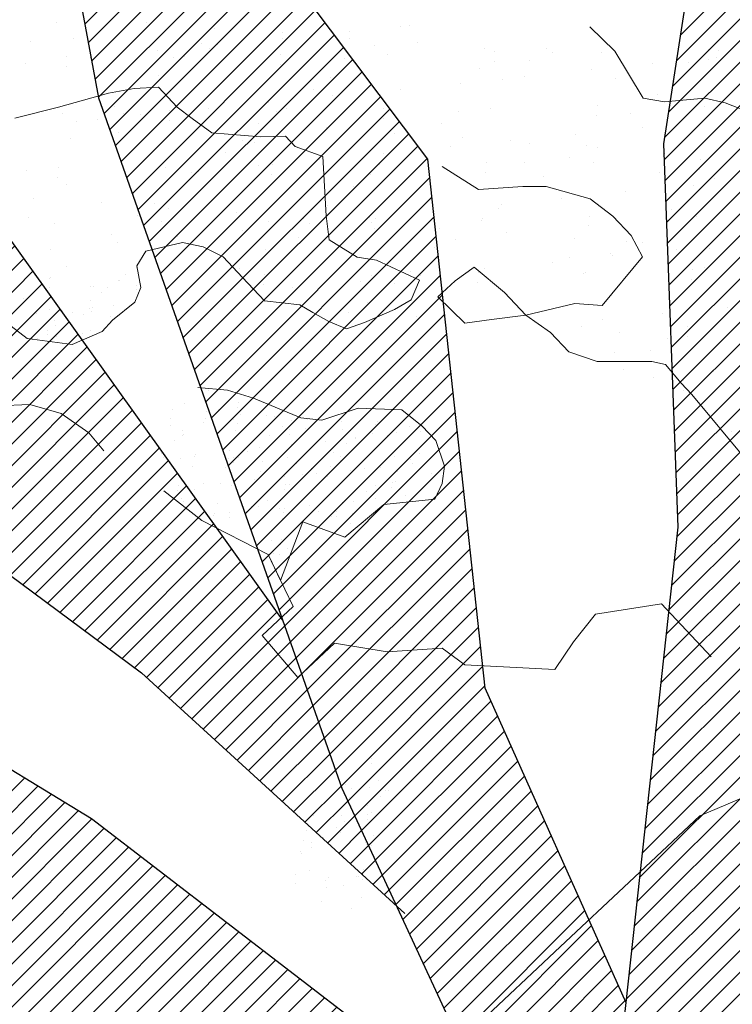
# Model space of a CAD drawing. Units: inches. Extents: x 1986 to 21484, y -1816 to 2016.
# Tile 72 of 85: x 3662.33 to 3669.485, y 1888.787 to 1898.672. Entities that reach past the tile are written whole.
import ezdxf

# ---------------------------------------------------------------- set-up
doc = ezdxf.new("R2010")
doc.units = ezdxf.units.IN
doc.layers.add('L-PLNT', color=84, linetype='Continuous', lineweight=13)
doc.layers.add('vfolhas', color=114, linetype='Continuous', lineweight=5)
doc.layers.add('vfolha2', color=110, linetype='Continuous')
doc.layers.add('vfolhas2', color=102, linetype='Continuous')
pattern_1 = [(45, (-2446.5133113, 50.986076), (-0.004419417382, 0.004419417382), [])]

# ---------------------------------------------------------------- blocks, each defined once
blk = doc.blocks.new('arbusto_PB_verde_grande')
at = {"layer": 'vfolha2'}
h = blk.add_hatch(dxfattribs=at)
h.set_pattern_fill('ANSI31', color=256, scale=0.05, style=0)
h.set_pattern_definition(pattern_1)
h.paths.add_polyline_path([(0.02944, 0.35651), (0.00028, 0.09048), (0.02625, -0.03934), (0.047, 0.06233), (0.06189, 0.09731), (0.09372, 0.26573), (0.09955, 0.43473), (0.08789, 0.61313), (0.0645, 0.72266), (0.04988, 0.6851), (0.0236, 0.51294)])
h.paths.add_polyline_path([(0.30106, 0.43789), (0.14225, 0.24871), (0.26685, 0.30022)])
h.paths.add_polyline_path([(0.37995, 0.22817), (0.23697, 0.15193), (0.18428, 0.09364), (0.11122, 0.04358), (0.02625, -0.03934), (0.28061, 0.04667), (0.36829, 0.07798), (0.46756, 0.11239), (0.61068, 0.19376), (0.71585, 0.27823), (0.55813, 0.25948)])
h.paths.add_polyline_path([(0.56101, -0.29441), (0.72752, -0.32573), (0.59024, -0.2412), (0.42962, -0.15982), (0.02625, -0.03934), (0.14922, -0.14107), (0.18838, -0.16604), (0.41501, -0.24435)])
h.paths.add_polyline_path([(-0.27429, -0.44776), (-0.30352, -0.72628), (-0.23923, -0.64175), (-0.15457, -0.45716), (0.02625, -0.03934), (-0.16328, -0.25376)])
h.paths.add_polyline_path([(-0.51963, -0.24744), (-0.67736, -0.32573), (-0.59558, -0.35072), (-0.40574, -0.32882), (-0.21007, -0.20995), (0.02625, -0.03934), (-0.14874, -0.06595), (-0.31518, -0.09101), (-0.41452, -0.15048)])
h.paths.add_polyline_path([(-0.52546, 0.25007), (-0.70947, 0.24698), (-0.51963, 0.1093), (-0.32979, 0.02167), (-0.07567, -0.0128), (-0.04234, -0.02148), (-0.35024, 0.1312)])
h = blk.add_hatch(dxfattribs=at)
h.set_pattern_fill('ANSI31', color=256, scale=0.05, style=0)
h.set_pattern_definition(pattern_1)
h.paths.add_polyline_path([(-0.18963, 0.29704), (-0.08553, 0.20192), (-0.10785, 0.25007), (-0.13202, 0.31865), (-0.25096, 0.48479), (-0.44952, 0.5505), (-0.37946, 0.43789)])
h.paths.add_polyline_path([(0.07911, -0.4071), (0.08214, -0.50631), (0.17255, -0.6355), (0.18428, -0.44151), (0.14904, -0.29177), (0.02625, -0.03934), (0.03527, -0.25376)])
at = {"layer": 'vfolhas'}
h = blk.add_hatch(dxfattribs=at)
h.set_pattern_fill('ANSI31', color=256, scale=0.05, style=0)
h.set_pattern_definition(pattern_1)
h.paths.add_polyline_path([(-0.07279, 0.50669), (-0.18085, 0.65063), (-0.2334, 0.67253), (-0.20712, 0.53176), (-0.10785, 0.25007), (0.02625, -0.03934), (0.00028, 0.09048), (0.00816, 0.16241), (-0.04939, 0.29079)])
h.paths.add_polyline_path([(0.09902, 0.41929), (0.09372, 0.26573), (0.07906, 0.18814), (0.15506, 0.36901), (0.26606, 0.5505), (0.28356, 0.63504), (0.2485, 0.68819), (0.25145, 0.63504), (0.20178, 0.54426)])
h.paths.add_polyline_path([(0.12295, 0.24073), (0.047, 0.06233), (0.02625, -0.03934), (0.11122, 0.04358), (0.18428, 0.09364), (0.27478, 0.19376), (0.3215, 0.25323), (0.44129, 0.38467), (0.47634, 0.57866), (0.41789, 0.45347), (0.28939, 0.30954)])
h.paths.add_polyline_path([(0.58145, -0.03779), (0.70707, 0.01536), (0.78591, 0.04667), (0.74796, 0.06549), (0.62818, 0.08423), (0.52595, 0.09048), (0.39745, 0.04358), (0.02625, -0.03934), (0.25728, -0.03154), (0.43834, -0.0347)])
h.paths.add_polyline_path([(0.52022, -0.03647), (0.43834, -0.0347), (0.25728, -0.03154), (0.02625, -0.03934), (0.17964, -0.08515), (0.53768, -0.13167), (0.69541, -0.15357), (0.78591, -0.07852), (0.70413, -0.10042)])
h.paths.add_polyline_path([(0.27189, -0.21929), (0.14922, -0.14107), (0.02625, -0.03934), (0.15794, -0.31007), (0.29522, -0.42585), (0.41789, -0.49157), (0.56396, -0.56669), (0.5114, -0.48532), (0.39456, -0.34139)])
h.paths.add_polyline_path([(-0.05818, -0.47591), (-0.02312, -0.61984), (0.047, -0.80134), (0.08494, -0.59794), (0.07911, -0.4071), (0.03527, -0.25376), (0.02625, -0.03934), (-0.03773, -0.26001)])
h.paths.add_polyline_path([(-0.24218, 0.14054), (-0.11073, 0.06858), (0.02625, -0.03934), (-0.04235, 0.10871), (-0.21007, 0.23757), (-0.36485, 0.33145), (-0.47874, 0.40341), (-0.54303, 0.46288), (-0.49041, 0.33145), (-0.39408, 0.22192)])
at = {"layer": 'vfolha2'}
for p, q in [((0.0236, 0.51294), (0.04988, 0.6851)), ((0.02944, 0.35651), (0.0236, 0.51294)), ((-0.13202, 0.31865), (-0.25096, 0.48479)), ((-0.37946, 0.43789), (-0.18963, 0.29704)), ((0.00028, 0.09048), (0.02944, 0.35651)), ((-0.18963, 0.29704), (-0.0822, 0.19888))]:
    blk.add_line(p, q, dxfattribs=at)
at = {"layer": 'vfolhas2'}
for p, q in [((-0.2334, 0.67253), (-0.20712, 0.53176)), ((-0.07279, 0.50669), (-0.18085, 0.65063)), ((-0.20712, 0.53176), (-0.10785, 0.25007)), ((-0.04939, 0.29079), (-0.07279, 0.50669)), ((-0.21007, 0.23757), (-0.36485, 0.33145)), ((0.00816, 0.16241), (-0.04939, 0.29079)), ((-0.10785, 0.25007), (0.02625, -0.03934)), ((-0.04235, 0.10871), (-0.21007, 0.23757))]:
    blk.add_line(p, q, dxfattribs=at)
blk = doc.blocks.new('PLANT-SHRUB')
for p, q in [((2158.5196, 1885.4461), (2159.249, 1885.1789)), ((2159.249, 1885.1789), (2160.2216, 1885.1789)), ((2160.2216, 1885.1789), (2161.1699, 1885.1789)), ((2161.1699, 1885.1789), (2162.4585, 1885.1789)), ((2158.073, 1884.091), (2158.073, 1883.3626)), ((2162.2901, 1883.45), (2162.2901, 1883.45)), ((2162.4393, 1883.4653), (2162.4393, 1883.4653)), ((2158.073, 1883.3626), (2158.626, 1882.9859)), ((2158.073, 1883.3626), (2158.073, 1883.3626)), ((2162.1557, 1883.33), (2162.1557, 1883.33)), ((2162.072, 1883.2774), (2162.072, 1883.2774)), ((2162.0794, 1883.2569), (2162.0794, 1883.2569)), ((2162.1162, 1883.2907), (2162.1162, 1883.2907)), ((2162.1691, 1883.2779), (2162.1691, 1883.2779)), ((2162.176, 1883.2637), (2162.176, 1883.2637)), ((2162.3385, 1883.2423), (2162.3385, 1883.2423)), ((2158.9779, 1883.0361), (2159.3046, 1883.1115)), ((2159.3046, 1883.1115), (2159.933, 1882.4585)), ((2159.3046, 1883.1115), (2159.3046, 1883.1115)), ((2159.3046, 1883.1115), (2159.3046, 1883.1115)), ((2161.8523, 1883.1367), (2161.8523, 1883.1367)), ((2162.4746, 1883.1356), (2162.4746, 1883.1356)), ((2162.6099, 1883.2066), (2162.6099, 1883.2066)), ((2158.626, 1882.9859), (2158.9779, 1883.0361)), ((2161.7681, 1883.083), (2161.7681, 1883.083)), ((2161.8805, 1883.0746), (2161.8805, 1883.0746)), ((2161.887, 1883.0997), (2161.887, 1883.0997)), ((2162.3904, 1883.0819), (2162.3904, 1883.0819)), ((2162.4267, 1883.0802), (2162.4267, 1883.0802)), ((2161.7066, 1882.9153), (2161.7066, 1882.9153)), ((2156.412, 1882.0396), (2156.4637, 1882.8912)), ((2161.3498, 1882.8551), (2161.3498, 1882.8551)), ((2161.372, 1882.8307), (2161.372, 1882.8307)), ((2161.4539, 1882.8414), (2161.4539, 1882.8414)), ((2161.6163, 1882.82), (2161.6163, 1882.82)), ((2161.6334, 1882.8995), (2161.6334, 1882.8995)), ((2161.6698, 1882.8816), (2161.6698, 1882.8816)), ((2161.9943, 1882.8296), (2161.9943, 1882.8296)), ((2162.1565, 1882.8928), (2162.1565, 1882.8928)), ((2162.4812, 1882.8993), (2162.4812, 1882.8993)), ((2162.6166, 1882.8284), (2162.6166, 1882.8284)), ((2162.6677, 1882.8953), (2162.6677, 1882.8953)), ((2161.8878, 1882.7842), (2161.8878, 1882.7842)), ((2161.9918, 1882.7705), (2161.9918, 1882.7705)), ((2162.1542, 1882.7492), (2162.1542, 1882.7492)), ((2162.3074, 1882.7399), (2162.3074, 1882.7399)), ((2161.3632, 1882.7122), (2161.3632, 1882.7122)), ((2161.4709, 1882.6993), (2161.4709, 1882.6993)), ((2161.6909, 1882.6363), (2161.6909, 1882.6363)), ((2161.8744, 1882.7146), (2161.8744, 1882.7146)), ((2162.2705, 1882.7062), (2162.2705, 1882.7062)), ((2162.3133, 1882.6352), (2162.3133, 1882.6352)), ((2162.4141, 1882.6952), (2162.4141, 1882.6952)), ((2162.4257, 1882.7134), (2162.4257, 1882.7134)), ((2156.3739, 1882.5863), (2156.3739, 1882.5863)), ((2161.297, 1882.54), (2161.297, 1882.54)), ((2161.6067, 1882.5826), (2161.6067, 1882.5826)), ((2162.0716, 1882.5239), (2162.0716, 1882.5239)), ((2162.229, 1882.5815), (2162.229, 1882.5815)), ((2159.933, 1882.4585), (2159.9833, 1882.1822)), ((2161.2602, 1882.5063), (2161.2602, 1882.5063)), ((2161.6208, 1882.5145), (2161.6208, 1882.5145)), ((2162.1439, 1882.5078), (2162.1439, 1882.5078)), ((2159.9833, 1882.1822), (2160.4105, 1881.8306)), ((2159.9833, 1882.1822), (2159.9833, 1882.1822)), ((2156.412, 1881.8848), (2156.412, 1882.0396)), ((2156.0929, 1882.0197), (2156.0929, 1882.0197)), ((2156.4461, 1881.9494), (2156.4461, 1881.9494)), ((2156.3724, 1881.8819), (2156.3724, 1881.8819)), ((2156.3991, 1881.6396), (2156.412, 1881.8848)), ((2160.4105, 1881.8306), (2160.7373, 1881.4037)), ((2160.4105, 1881.8306), (2160.4105, 1881.8306)), ((2155.5524, 1881.645), (2155.5524, 1881.645)), ((2156.4766, 1881.5235), (2156.3991, 1881.6396)), ((2156.5748, 1881.6499), (2156.5748, 1881.6499)), ((2155.6627, 1881.5342), (2155.6627, 1881.5342)), ((2156.0511, 1881.5855), (2156.0511, 1881.5855)), ((2155.9746, 1881.5174), (2155.9746, 1881.5174)), ((2156.2055, 1881.4627), (2156.2055, 1881.4627)), ((2156.4136, 1881.4353), (2156.4136, 1881.4353)), ((2156.4766, 1881.5235), (2156.8784, 1881.1488)), ((2156.7385, 1881.3925), (2156.7385, 1881.3925)), ((2160.7373, 1881.4037), (2161.24, 1881.4037)), ((2161.24, 1881.4037), (2161.2149, 1880.8511)), ((2154.164, 1880.1332), (2153.6083, 1881.3076)), ((2156.0677, 1881.2496), (2156.0677, 1881.2496)), ((2155.4444, 1881.1989), (2155.4444, 1881.1989)), ((2155.6269, 1881.1988), (2155.6269, 1881.1988)), ((2156.689, 1881.1967), (2156.689, 1881.1967)), ((2156.8784, 1881.1488), (2157.0196, 1880.8823)), ((2155.2758, 1881.0916), (2155.2758, 1881.0916)), ((2155.5532, 1881.1313), (2155.5532, 1881.1313)), ((2156.5205, 1881.0893), (2156.5205, 1881.0893)), ((2159.0126, 1881.0382), (2158.8512, 1880.9762)), ((2159.4223, 1880.7281), (2159.0126, 1881.0382)), ((2158.8512, 1880.9762), (2158.7146, 1880.8646)), ((2155.5273, 1880.8749), (2155.5273, 1880.8749)), ((2156.5497, 1880.8798), (2156.5497, 1880.8798)), ((2157.0196, 1880.8823), (2157.0196, 1880.6157)), ((2158.7146, 1880.8646), (2158.6029, 1880.6164)), ((2160.7876, 1880.8511), (2160.6116, 1880.2986)), ((2161.2149, 1880.8511), (2160.7876, 1880.8511)), ((2155.1554, 1880.7668), (2155.1554, 1880.7668)), ((2156.4547, 1880.7725), (2155.8271, 1880.6941)), ((2156.643, 1880.5687), (2156.4547, 1880.7725)), ((2156.7547, 1880.7805), (2156.7547, 1880.7805)), ((2158.8595, 1880.8325), (2158.8595, 1880.8325)), ((2159.2032, 1880.8173), (2159.2032, 1880.8173)), ((2155.8271, 1880.6941), (2155.7643, 1880.4589)), ((2159.2491, 1880.6634), (2159.2491, 1880.6634)), ((2159.933, 1880.7004), (2159.4223, 1880.7281)), ((2159.933, 1880.7004), (2159.933, 1880.7004)), ((2160.1341, 1880.2986), (2159.933, 1880.7004)), ((2154.7612, 1880.618), (2154.7612, 1880.618)), ((2154.9693, 1880.5906), (2154.9693, 1880.5906)), ((2155.2942, 1880.5479), (2155.2942, 1880.5479)), ((2155.7283, 1880.5847), (2155.7283, 1880.5847)), ((2157.0823, 1880.3178), (2156.643, 1880.5687)), ((2157.0196, 1880.6157), (2157.0823, 1880.3178)), ((2158.6029, 1880.6164), (2158.6029, 1880.4179)), ((2158.8149, 1880.6018), (2158.8149, 1880.6018)), ((2158.9189, 1880.5881), (2158.9189, 1880.5881)), ((2158.9329, 1880.6299), (2158.9329, 1880.6299)), ((2159.0813, 1880.5667), (2159.0813, 1880.5667)), ((2159.0941, 1880.5844), (2159.0941, 1880.5844)), ((2159.1784, 1880.6381), (2159.1784, 1880.6381)), ((2159.2123, 1880.6297), (2159.2123, 1880.6297)), ((2159.4441, 1880.6323), (2159.4441, 1880.6323)), ((2159.7165, 1880.5832), (2159.7165, 1880.5832)), ((2159.8007, 1880.6369), (2159.8007, 1880.6369)), ((2160.6996, 1880.5749), (2160.1341, 1880.2986)), ((2160.6116, 1880.2986), (2160.6996, 1880.5749)), ((2160.6996, 1880.5749), (2160.6996, 1880.5749)), ((2154.8077, 1880.4482), (2154.8077, 1880.4482)), ((2154.9631, 1880.5184), (2154.9631, 1880.5184)), ((2155.7643, 1880.4589), (2155.7643, 1880.1924)), ((2155.837, 1880.4764), (2155.837, 1880.4764)), ((2156.0425, 1880.4795), (2156.0425, 1880.4795)), ((2156.0451, 1880.449), (2156.0451, 1880.449)), ((2158.6508, 1880.4516), (2158.6508, 1880.4516)), ((2159.0134, 1880.4474), (2159.0134, 1880.4474)), ((2159.3528, 1880.5309), (2159.3528, 1880.5309)), ((2159.4568, 1880.5173), (2159.4568, 1880.5173)), ((2159.6193, 1880.4959), (2159.6193, 1880.4959)), ((2159.813, 1880.4543), (2159.813, 1880.4543)), ((2159.8498, 1880.488), (2159.8498, 1880.488)), ((2159.8907, 1880.4601), (2159.8907, 1880.4601)), ((2159.9947, 1880.4464), (2159.9947, 1880.4464)), ((2160.6244, 1880.472), (2160.6244, 1880.472)), ((2154.734, 1880.3807), (2154.734, 1880.3807)), ((2156.3569, 1880.416), (2156.3569, 1880.416)), ((2156.37, 1880.4062), (2156.37, 1880.4062)), ((2158.6029, 1880.4179), (2158.6401, 1880.1574)), ((2159.1906, 1880.4322), (2159.1906, 1880.4322)), ((2159.7137, 1880.4255), (2159.7137, 1880.4255)), ((2160.4286, 1880.3893), (2160.4286, 1880.3893)), ((2160.5326, 1880.3756), (2160.5326, 1880.3756)), ((2157.0823, 1880.0043), (2157.0823, 1880.3178)), ((2157.0823, 1880.3178), (2157.3648, 1880.114)), ((2158.6981, 1880.3321), (2158.6981, 1880.3321)), ((2158.8027, 1880.2544), (2158.8027, 1880.2544)), ((2158.8395, 1880.2881), (2158.8395, 1880.2881)), ((2158.9203, 1880.2448), (2158.9203, 1880.2448)), ((2159.3204, 1880.3309), (2159.3204, 1880.3309)), ((2159.4315, 1880.2473), (2159.4315, 1880.2473)), ((2159.6141, 1880.272), (2159.6141, 1880.272)), ((2159.9427, 1880.3298), (2159.9427, 1880.3298)), ((2160.1341, 1880.2986), (2160.1341, 1880.2986)), ((2160.4137, 1880.2789), (2160.4137, 1880.2789)), ((2160.4506, 1880.3126), (2160.4506, 1880.3126)), ((2160.565, 1880.3287), (2160.565, 1880.3287)), ((2160.6116, 1880.2986), (2160.863, 1879.5954)), ((2160.6116, 1880.2986), (2160.6116, 1880.2986)), ((2155.1216, 1880.1981), (2155.1216, 1880.1981)), ((2155.7643, 1880.1924), (2155.8114, 1879.9102)), ((2156.3662, 1880.1959), (2156.3662, 1880.1959)), ((2158.6401, 1880.1574), (2158.9505, 1879.8472)), ((2159.9713, 1880.2278), (2159.9713, 1880.2278)), ((2160.4944, 1880.2212), (2160.4944, 1880.2212)), ((2154.2807, 1879.9584), (2154.164, 1880.1332)), ((2154.4559, 1880.1182), (2154.4559, 1880.1182)), ((2154.9531, 1880.0908), (2154.9531, 1880.0908)), ((2155.5021, 1880.1048), (2155.5021, 1880.1048)), ((2156.0092, 1880.0974), (2156.0092, 1880.0974)), ((2156.1977, 1880.0885), (2156.1977, 1880.0885)), ((2156.5245, 1880.1097), (2156.5245, 1880.1097)), ((2157.3648, 1880.114), (2157.5844, 1879.9572)), ((2158.7346, 1880.0949), (2158.7346, 1880.0949)), ((2158.8971, 1880.0735), (2158.8971, 1880.0735)), ((2158.9328, 1880.084), (2158.9328, 1880.084)), ((2159.017, 1880.1377), (2159.017, 1880.1377)), ((2159.178, 1880.0472), (2159.178, 1880.0472)), ((2159.4034, 1880.079), (2159.4034, 1880.079)), ((2159.4402, 1880.1127), (2159.4402, 1880.1127)), ((2159.5551, 1880.0828), (2159.5551, 1880.0828)), ((2159.6393, 1880.1365), (2159.6393, 1880.1365)), ((2160.1774, 1880.0817), (2160.1774, 1880.0817)), ((2160.2148, 1880.0966), (2160.2148, 1880.0966)), ((2160.2617, 1880.1354), (2160.2617, 1880.1354)), ((2154.6015, 1879.7107), (2154.2807, 1879.9584)), ((2154.3362, 1880.0161), (2154.3362, 1880.0161)), ((2155.9355, 1880.0299), (2155.9355, 1880.0299)), ((2157.1294, 1879.6123), (2157.0823, 1880.0043)), ((2157.5844, 1879.9572), (2157.6001, 1879.5809)), ((2157.5844, 1879.9572), (2157.5844, 1879.9572)), ((2159.1685, 1880.0378), (2159.1685, 1880.0378)), ((2159.2725, 1880.0241), (2159.2725, 1880.0241)), ((2159.435, 1880.0027), (2159.435, 1880.0027)), ((2159.7011, 1880.0405), (2159.7011, 1880.0405)), ((2159.7064, 1879.967), (2159.7064, 1879.967)), ((2159.8105, 1879.9533), (2159.8105, 1879.9533)), ((2160.2123, 1880.0429), (2160.2123, 1880.0429)), ((2155.8114, 1879.9102), (2156.0496, 1879.5165)), ((2159.2045, 1879.8967), (2159.2045, 1879.8967)), ((2159.419, 1879.8622), (2159.419, 1879.8622)), ((2159.9729, 1879.9319), (2159.9729, 1879.9319)), ((2160.0041, 1879.9036), (2160.0041, 1879.9036)), ((2160.041, 1879.9373), (2160.041, 1879.9373)), ((2160.2444, 1879.8962), (2160.2444, 1879.8962)), ((2160.3484, 1879.8825), (2160.3484, 1879.8825)), ((2160.5108, 1879.8611), (2160.5108, 1879.8611)), ((2158.9505, 1879.8472), (2159.2982, 1879.686)), ((2159.159, 1879.8305), (2159.159, 1879.8305)), ((2159.7813, 1879.8294), (2159.7813, 1879.8294)), ((2159.9587, 1879.8428), (2159.9587, 1879.8428)), ((2160.4036, 1879.8283), (2160.4036, 1879.8283)), ((2160.4818, 1879.8361), (2160.4818, 1879.8361)), ((2160.6417, 1879.7619), (2160.6417, 1879.7619)), ((2153.8499, 1879.7032), (2153.8499, 1879.7032)), ((2153.9155, 1879.7434), (2153.9155, 1879.7434)), ((2153.9885, 1879.6975), (2153.9885, 1879.6975)), ((2154.7327, 1879.5359), (2154.6015, 1879.7107)), ((2154.9379, 1879.7483), (2154.9379, 1879.7483)), ((2155.5377, 1879.6654), (2155.5377, 1879.6654)), ((2156.0173, 1879.7094), (2156.0173, 1879.7094)), ((2157.0635, 1879.6961), (2157.0635, 1879.6961)), ((2157.137, 1879.6791), (2157.137, 1879.6791)), ((2157.2106, 1879.7466), (2157.2106, 1879.7466)), ((2159.2982, 1879.686), (2159.4348, 1879.5247)), ((2159.6885, 1879.6554), (2159.6885, 1879.6554)), ((2159.8052, 1879.7213), (2159.8052, 1879.7213)), ((2160.1997, 1879.6579), (2160.1997, 1879.6579)), ((2160.6049, 1879.7282), (2160.6049, 1879.7282)), ((2153.9149, 1879.63), (2153.9149, 1879.63)), ((2154.1609, 1879.5861), (2154.1609, 1879.5861)), ((2154.3927, 1879.6317), (2154.3927, 1879.6317)), ((2154.6008, 1879.6044), (2154.6008, 1879.6044)), ((2154.9257, 1879.5616), (2154.9257, 1879.5616)), ((2155.4056, 1879.5838), (2155.4056, 1879.5838)), ((2156.6502, 1879.5816), (2156.6502, 1879.5816)), ((2157.3648, 1879.5809), (2157.1294, 1879.6123)), ((2157.6001, 1879.5809), (2157.3648, 1879.5809)), ((2157.8948, 1879.5793), (2157.8948, 1879.5793)), ((2159.3937, 1879.5824), (2159.3937, 1879.5824)), ((2159.4779, 1879.6361), (2159.4779, 1879.6361)), ((2159.6314, 1879.562), (2159.6314, 1879.562)), ((2160.016, 1879.5813), (2160.016, 1879.5813)), ((2160.1003, 1879.635), (2160.1003, 1879.635)), ((2160.6383, 1879.5802), (2160.6383, 1879.5802)), ((2160.7226, 1879.6339), (2160.7226, 1879.6339)), ((2160.7394, 1879.6384), (2160.7394, 1879.6384)), ((2160.863, 1879.5954), (2160.9384, 1879.1182)), ((2154.6161, 1878.9968), (2154.7327, 1879.5359)), ((2155.4685, 1879.4901), (2155.4685, 1879.4901)), ((2155.6766, 1879.4627), (2155.6766, 1879.4627)), ((2156.0496, 1879.5165), (2156.2178, 1879.3557)), ((2159.4348, 1879.5247), (2159.6458, 1879.0532)), ((2159.4348, 1879.5247), (2159.4348, 1879.5247)), ((2159.5222, 1879.4738), (2159.5222, 1879.4738)), ((2159.5945, 1879.5283), (2159.5945, 1879.5283)), ((2159.6262, 1879.4601), (2159.6262, 1879.4601)), ((2159.9461, 1879.4578), (2159.9461, 1879.4578)), ((2160.406, 1879.5459), (2160.406, 1879.5459)), ((2156.0015, 1879.4199), (2156.0015, 1879.4199)), ((2156.2178, 1879.3557), (2156.5647, 1879.0723)), ((2157.6195, 1879.3297), (2157.8177, 1879.4177)), ((2157.8177, 1879.4177), (2158.0049, 1879.3737)), ((2158.0049, 1879.3737), (2158.3132, 1879.2637)), ((2159.7887, 1879.4388), (2159.7887, 1879.4388)), ((2160.0601, 1879.403), (2160.0601, 1879.403)), ((2160.1641, 1879.3893), (2160.1641, 1879.3893)), ((2160.2321, 1879.3866), (2160.2321, 1879.3866)), ((2160.3266, 1879.3679), (2160.3266, 1879.3679)), ((2160.4692, 1879.4511), (2160.4692, 1879.4511)), ((2154.4307, 1879.3481), (2154.4307, 1879.3481)), ((2155.1163, 1879.2792), (2155.1163, 1879.2792)), ((2155.19, 1879.3468), (2155.19, 1879.3468)), ((2155.4769, 1879.3347), (2155.4769, 1879.3347)), ((2156.4993, 1879.3396), (2156.4993, 1879.3396)), ((2156.5444, 1879.3485), (2156.5444, 1879.3485)), ((2156.7392, 1879.3146), (2156.7392, 1879.3146)), ((2156.7524, 1879.3211), (2156.7524, 1879.3211)), ((2157.0773, 1879.2783), (2157.0773, 1879.2783)), ((2157.5788, 1879.3007), (2157.5788, 1879.3007)), ((2157.7956, 1878.8896), (2157.6195, 1879.3297)), ((2158.3132, 1879.2637), (2158.4894, 1879.1867)), ((2159.6199, 1879.329), (2159.6199, 1879.329)), ((2159.6759, 1879.2704), (2159.6759, 1879.2704)), ((2160.1871, 1879.2728), (2160.1871, 1879.2728)), ((2160.1953, 1879.3529), (2160.1953, 1879.3529)), ((2160.2422, 1879.3278), (2160.2422, 1879.3278)), ((2160.598, 1879.3322), (2160.598, 1879.3322)), ((2160.702, 1879.3185), (2160.702, 1879.3185)), ((2160.8645, 1879.2971), (2160.8645, 1879.2971)), ((2160.8646, 1879.3267), (2160.8646, 1879.3267)), ((2154.7988, 1879.1973), (2154.7988, 1879.1973)), ((2156.0434, 1879.195), (2156.0434, 1879.195)), ((2157.2881, 1879.1928), (2157.2881, 1879.1928)), ((2157.6202, 1879.2068), (2157.6202, 1879.2068)), ((2157.8282, 1879.1794), (2157.8282, 1879.1794)), ((2158.4894, 1879.1867), (2158.5664, 1879.0106)), ((2159.9964, 1879.1706), (2159.9964, 1879.1706)), ((2160.7268, 1879.2534), (2160.7268, 1879.2534)), ((2160.796, 1879.1775), (2160.796, 1879.1775)), ((2160.8328, 1879.2112), (2160.8328, 1879.2112)), ((2154.6303, 1879.0899), (2154.6303, 1879.0899)), ((2155.8749, 1879.0877), (2155.8749, 1879.0877)), ((2156.5647, 1879.0723), (2156.6744, 1878.6559)), ((2157.1195, 1879.0854), (2157.1195, 1879.0854)), ((2158.1532, 1879.1367), (2158.1532, 1879.1367)), ((2158.3642, 1879.0832), (2158.3642, 1879.0832)), ((2159.8546, 1879.0809), (2159.8546, 1879.0809)), ((2159.9335, 1879.0727), (2159.9335, 1879.0727)), ((2159.9389, 1879.1346), (2159.9389, 1879.1346)), ((2160.4566, 1879.066), (2160.4566, 1879.066)), ((2160.4769, 1879.0798), (2160.4769, 1879.0798)), ((2160.5612, 1879.1334), (2160.5612, 1879.1334)), ((2154.6306, 1878.6471), (2154.6161, 1878.9968)), ((2154.9127, 1878.9782), (2154.9127, 1878.9782)), ((2156.3915, 1878.996), (2156.3915, 1878.996)), ((2157.9406, 1878.9638), (2157.9406, 1878.9638)), ((2158.5664, 1879.0106), (2158.6215, 1878.8346)), ((2159.6458, 1879.0532), (2159.7824, 1878.8175)), ((2159.7857, 1878.9775), (2159.7857, 1878.9775)), ((2159.8225, 1879.0113), (2159.8225, 1879.0113)), ((2160.5971, 1878.9952), (2160.5971, 1878.9952)), ((2154.7185, 1878.9147), (2154.7185, 1878.9147)), ((2155.9922, 1878.9393), (2155.9922, 1878.9393)), ((2156.3178, 1878.9285), (2156.3178, 1878.9285)), ((2157.0383, 1878.926), (2157.0383, 1878.926)), ((2157.9168, 1878.7356), (2157.7956, 1878.8896)), ((2158.0607, 1878.9309), (2158.0607, 1878.9309)), ((2159.8759, 1878.9099), (2159.8759, 1878.9099)), ((2159.9799, 1878.8962), (2159.9799, 1878.8962)), ((2160.1423, 1878.8748), (2160.1423, 1878.8748)), ((2160.1745, 1878.8878), (2160.1745, 1878.8878)), ((2160.7142, 1878.8683), (2160.7142, 1878.8683)), ((2158.6215, 1878.8346), (2158.6655, 1878.6916)), ((2159.7824, 1878.8175), (2159.9811, 1878.5942)), ((2160.0809, 1878.8274), (2160.0809, 1878.8274)), ((2160.3864, 1878.8022), (2160.3864, 1878.8022)), ((2160.4138, 1878.8391), (2160.4138, 1878.8391)), ((2160.4233, 1878.8359), (2160.4233, 1878.8359)), ((2160.5178, 1878.8254), (2160.5178, 1878.8254)), ((2160.6803, 1878.804), (2160.6803, 1878.804)), ((2160.7032, 1878.8263), (2160.7032, 1878.8263)), ((2158.0049, 1878.4165), (2157.9168, 1878.7356)), ((2158.6655, 1878.6916), (2158.8968, 1878.4165)), ((2159.9209, 1878.6877), (2159.9209, 1878.6877)), ((2160.444, 1878.681), (2160.444, 1878.681)), ((2155.0828, 1878.583), (2155.0828, 1878.583)), ((2155.4517, 1878.5646), (2155.4517, 1878.5646)), ((2155.92, 1878.5639), (2155.92, 1878.5639)), ((2156.3274, 1878.5808), (2156.3274, 1878.5808)), ((2156.4741, 1878.5695), (2156.4741, 1878.5695)), ((2157.5193, 1878.5777), (2157.5193, 1878.5777)), ((2157.572, 1878.5785), (2157.572, 1878.5785)), ((2157.5929, 1878.6452), (2157.5929, 1878.6452)), ((2159.9811, 1878.5942), (2159.9811, 1878.5942)), ((2160.1875, 1878.6199), (2160.1875, 1878.6199)), ((2160.3155, 1878.5794), (2160.3155, 1878.5794)), ((2160.3998, 1878.633), (2160.3998, 1878.633)), ((2155.1001, 1878.5038), (2155.1001, 1878.5038)), ((2155.3081, 1878.4764), (2155.3081, 1878.4764)), ((2157.5536, 1878.5306), (2157.5536, 1878.5306)), ((2158.5998, 1878.5173), (2158.5998, 1878.5173)), ((2155.633, 1878.4336), (2155.633, 1878.4336)), ((2157.8617, 1878.2184), (2158.0049, 1878.4165)), ((2158.0049, 1878.4165), (2158.0049, 1878.4165)), ((2158.8968, 1878.4165), (2158.8968, 1878.0974)), ((2161.1044, 1878.4126), (2161.0905, 1878.1766)), ((2156.1759, 1878.3622), (2156.1759, 1878.3622)), ((2156.3839, 1878.3348), (2156.3839, 1878.3348)), ((2156.7088, 1878.292), (2156.7088, 1878.292)), ((2158.7944, 1878.2944), (2158.7944, 1878.2944)), ((2155.4986, 1878.1778), (2155.4986, 1878.1778)), ((2155.5723, 1878.2453), (2155.5723, 1878.2453)), ((2155.7207, 1878.1942), (2155.7207, 1878.1942)), ((2155.967, 1878.1692), (2155.967, 1878.1692)), ((2156.9653, 1878.192), (2156.9653, 1878.192)), ((2157.1215, 1878.2132), (2157.1215, 1878.2132)), ((2157.2517, 1878.2205), (2157.2517, 1878.2205)), ((2157.4597, 1878.1932), (2157.4597, 1878.1932)), ((2157.4779, 1877.7629), (2157.8617, 1878.2184)), ((2158.2099, 1878.1897), (2158.2099, 1878.1897)), ((2158.7207, 1878.2269), (2158.7207, 1878.2269)), ((2161.0905, 1878.1766), (2161.1599, 1877.8434)), ((2155.5521, 1878.0869), (2155.5521, 1878.0869)), ((2156.7968, 1878.0846), (2156.7968, 1878.0846)), ((2157.0132, 1878.1559), (2157.0132, 1878.1559)), ((2157.7847, 1878.1504), (2157.7847, 1878.1504)), ((2158.0356, 1878.1608), (2158.0356, 1878.1608)), ((2158.0414, 1878.0823), (2158.0414, 1878.0823)), ((2158.3275, 1878.0789), (2158.3275, 1878.0789)), ((2158.8968, 1878.0974), (2158.8968, 1877.8113)), ((2158.5356, 1878.0515), (2158.5356, 1878.0515)), ((2158.8605, 1878.0087), (2158.8605, 1878.0087)), ((2156.7737, 1877.8946), (2156.7737, 1877.8946)), ((2156.449, 1877.7994), (2156.449, 1877.7994)), ((2156.7001, 1877.827), (2156.7001, 1877.827)), ((2158.3229, 1877.8624), (2158.3229, 1877.8624)), ((2158.8968, 1877.8113), (2158.9739, 1877.6023)), ((2161.1599, 1877.8434), (2161.3267, 1877.5657)), ((2157.61, 1877.4988), (2157.4779, 1877.7629)), ((2157.5284, 1877.7605), (2157.5284, 1877.7605)), ((2158.5746, 1877.7472), (2158.5746, 1877.7472)), ((2156.0046, 1877.58), (2156.0046, 1877.58)), ((2157.2493, 1877.5777), (2157.2493, 1877.5777)), ((2158.4939, 1877.5754), (2158.4939, 1877.5754)), ((2158.9739, 1877.6023), (2159.095, 1877.4262)), ((2157.61, 1877.3558), (2157.61, 1877.4988)), ((2157.9015, 1877.4763), (2157.9015, 1877.4763)), ((2157.9752, 1877.5438), (2157.9752, 1877.5438)), ((2159.7116, 1877.4703), (2159.8548, 1877.5363)), ((2159.8548, 1877.5363), (2160.1411, 1877.5143)), ((2160.1341, 1877.4782), (2160.1341, 1877.4782)), ((2160.1411, 1877.5143), (2160.2952, 1877.5253)), ((2160.1411, 1877.5143), (2160.1411, 1877.5143)), ((2160.2952, 1877.5253), (2160.6035, 1877.4152)), ((2161.3267, 1877.5657), (2161.6462, 1877.2881)), ((2155.9418, 1877.3992), (2155.9418, 1877.3992)), ((2156.3023, 1877.4625), (2156.3023, 1877.4625)), ((2156.988, 1877.3858), (2156.988, 1877.3858)), ((2158.0104, 1877.3907), (2158.0104, 1877.3907)), ((2159.095, 1877.4262), (2159.4253, 1877.2392)), ((2159.5905, 1877.2832), (2159.7116, 1877.4703)), ((2159.7256, 1877.4257), (2159.7256, 1877.4257)), ((2159.7551, 1877.4527), (2159.7551, 1877.4527)), ((2160.0368, 1877.4146), (2160.0368, 1877.4146)), ((2160.3748, 1877.4399), (2160.3748, 1877.4399)), ((2160.4553, 1877.4093), (2160.4553, 1877.4093)), ((2160.6035, 1877.4152), (2160.8925, 1877.0609)), ((2156.0154, 1877.3485), (2156.0154, 1877.3485)), ((2156.3403, 1877.3057), (2156.3403, 1877.3057)), ((2157.7972, 1877.1907), (2157.61, 1877.3558)), ((2159.0899, 1877.3518), (2159.0899, 1877.3518)), ((2159.4253, 1877.2392), (2159.5905, 1877.2832)), ((2159.6054, 1877.2898), (2159.6054, 1877.2898)), ((2160.2062, 1877.2854), (2160.2062, 1877.2854)), ((2160.2357, 1877.3124), (2160.2357, 1877.3124)), ((2156.6425, 1877.1912), (2156.6425, 1877.1912)), ((2156.8832, 1877.2342), (2156.8832, 1877.2342)), ((2157.0912, 1877.2069), (2157.0912, 1877.2069)), ((2158.1275, 1876.8277), (2157.7972, 1877.1907)), ((2157.8871, 1877.1889), (2157.8871, 1877.1889)), ((2159.1318, 1877.1866), (2159.1318, 1877.1866)), ((2159.1767, 1877.193), (2159.1767, 1877.193)), ((2159.4253, 1877.2392), (2159.4253, 1877.2392)), ((2159.7354, 1877.2727), (2159.7354, 1877.2727)), ((2159.8172, 1877.2764), (2159.8172, 1877.2764)), ((2159.8206, 1877.2647), (2159.8206, 1877.2647)), ((2159.9526, 1877.2441), (2159.9526, 1877.2441)), ((2160.0358, 1877.2331), (2160.0358, 1877.2331)), ((2160.1657, 1877.216), (2160.1657, 1877.216)), ((2160.2296, 1877.2667), (2160.2296, 1877.2667)), ((2160.3151, 1877.2755), (2160.3151, 1877.2755)), ((2160.3829, 1877.1874), (2160.3829, 1877.1874)), ((2160.6614, 1877.2511), (2160.6614, 1877.2511)), ((2156.474, 1877.0838), (2156.474, 1877.0838)), ((2157.4162, 1877.1641), (2157.4162, 1877.1641)), ((2157.5037, 1877.1117), (2157.5037, 1877.1117)), ((2157.7186, 1877.0815), (2157.7186, 1877.0815)), ((2157.959, 1877.0926), (2157.959, 1877.0926)), ((2159.103, 1877.1255), (2159.103, 1877.1255)), ((2160.0471, 1877.1396), (2160.0471, 1877.1396)), ((2160.0724, 1877.1208), (2160.0724, 1877.1208)), ((2160.4452, 1877.1013), (2160.4452, 1877.1013)), ((2160.4661, 1877.1765), (2160.4661, 1877.1765)), ((2160.5702, 1877.1199), (2160.5702, 1877.1199)), ((2160.5961, 1877.1594), (2160.5961, 1877.1594)), ((2160.6868, 1877.1451), (2160.6868, 1877.1451)), ((2160.7163, 1877.1721), (2160.7163, 1877.1721)), ((2160.8132, 1877.1308), (2160.8132, 1877.1308)), ((2160.8541, 1877.1032), (2160.8541, 1877.1032)), ((2156.4238, 1877.0293), (2156.4238, 1877.0293)), ((2157.5032, 1876.9904), (2157.5032, 1876.9904)), ((2158.1671, 1877.0652), (2158.1671, 1877.0652)), ((2158.492, 1877.0224), (2158.492, 1877.0224)), ((2158.9632, 1877.0793), (2158.9632, 1877.0793)), ((2159.5718, 1876.982), (2159.5718, 1876.982)), ((2160.5028, 1877.077), (2160.5028, 1877.077)), ((2160.5277, 1876.9993), (2160.5277, 1876.9993)), ((2160.8925, 1877.0609), (2160.9255, 1876.8629)), ((2158.5494, 1876.9771), (2158.5494, 1876.9771)), ((2159.0349, 1876.951), (2159.0349, 1876.951)), ((2159.2429, 1876.9236), (2159.2429, 1876.9236)), ((2160.6513, 1876.9431), (2160.6513, 1876.9431)), ((2157.156, 1876.7931), (2157.156, 1876.7931)), ((2158.1275, 1876.8277), (2158.1275, 1876.8277)), ((2158.1716, 1876.5856), (2158.1275, 1876.8277)), ((2159.5678, 1876.8808), (2159.5678, 1876.8808)), ((2160.1107, 1876.8093), (2160.1107, 1876.8093)), ((2160.3781, 1876.8422), (2160.3781, 1876.8422)), ((2157.0824, 1876.7256), (2157.0824, 1876.7256)), ((2158.7052, 1876.761), (2158.7052, 1876.761)), ((2160.3045, 1876.7747), (2160.3045, 1876.7747)), ((2160.3187, 1876.782), (2160.3187, 1876.782)), ((2160.6436, 1876.7392), (2160.6436, 1876.7392)), ((2156.9628, 1876.6157), (2156.9628, 1876.6157)), ((2157.9852, 1876.6206), (2157.9852, 1876.6206)), ((2156.9265, 1876.5769), (2156.9265, 1876.5769)), ((2158.1711, 1876.5746), (2158.1711, 1876.5746)), ((2158.2046, 1876.3985), (2158.1716, 1876.5856)), ((2159.0647, 1876.5817), (2159.0647, 1876.5817)), ((2159.4157, 1876.5723), (2159.4157, 1876.5723)), ((2160.1109, 1876.5684), (2160.1109, 1876.5684)), ((2158.2046, 1876.1235), (2158.2046, 1876.3985)), ((2158.3575, 1876.4423), (2158.3575, 1876.4423)), ((2159.9067, 1876.4102), (2159.9067, 1876.4102)), ((2158.2838, 1876.3748), (2158.2838, 1876.3748)), ((2157.4781, 1876.2203), (2157.4781, 1876.2203)), ((2158.5242, 1876.207), (2158.5242, 1876.207)), ((2159.5466, 1876.2119), (2159.5466, 1876.2119)), ((2157.5644, 1876.1881), (2157.5644, 1876.1881)), ((2157.5905, 1876.1063), (2157.5905, 1876.1063)), ((2158.3918, 1875.9694), (2158.2046, 1876.1235)), ((2158.809, 1876.1858), (2158.809, 1876.1858)), ((2160.0536, 1876.1836), (2160.0536, 1876.1836)), ((2157.3958, 1876.0807), (2157.3958, 1876.0807)), ((2157.7986, 1876.0789), (2157.7986, 1876.0789)), ((2157.886, 1876.0103), (2157.886, 1876.0103)), ((2158.1235, 1876.0361), (2158.1235, 1876.0361)), ((2158.6404, 1876.0784), (2158.6404, 1876.0784)), ((2159.4853, 1876.0241), (2159.4853, 1876.0241)), ((2159.559, 1876.0916), (2159.559, 1876.0916)), ((2159.8851, 1876.0762), (2159.8851, 1876.0762)), ((2158.612, 1875.8264), (2158.3918, 1875.9694)), ((2158.6664, 1875.9647), (2158.6664, 1875.9647)), ((2158.8744, 1875.9373), (2158.8744, 1875.9373)), ((2157.96, 1875.8505), (2157.96, 1875.8505)), ((2159.0745, 1875.5843), (2158.612, 1875.8264)), ((2159.0395, 1875.8116), (2159.0395, 1875.8116)), ((2159.1993, 1875.8945), (2159.1993, 1875.8945)), ((2159.7422, 1875.823), (2159.7422, 1875.823)), ((2159.0875, 1875.6595), (2159.0875, 1875.6595)), ((2157.8483, 1875.5738), (2157.8483, 1875.5738)), ((2159.0745, 1875.5843), (2159.0745, 1875.5843)), ((2159.4709, 1875.3643), (2159.0745, 1875.5843)), ((2159.0929, 1875.5715), (2159.0929, 1875.5715)), ((2158.4991, 1875.4369), (2158.4991, 1875.4369)), ((2158.7398, 1875.3409), (2158.7398, 1875.3409)), ((2158.6661, 1875.2734), (2158.6661, 1875.2734)), ((2158.4862, 1875.185), (2158.4862, 1875.185)), ((2159.0143, 1875.0415), (2159.0143, 1875.0415)), ((2158.5059, 1874.951), (2158.5059, 1874.951)), ((2158.8308, 1874.9082), (2158.8308, 1874.9082))]:
    blk.add_line(p, q)

msp = doc.modelspace()

# ---------------------------------------------------------------- block references
at = {"layer": 'L-PLNT', "rotation": 223.1883365522388}
msp.add_blockref('PLANT-SHRUB', (3953.27, 4742.9646), dxfattribs=at)
at = {"layer": 'L-PLNT', "xscale": 24.60366729364114, "yscale": 24.60366729364114, "zscale": 24.60366729364114}
msp.add_blockref('arbusto_PB_verde_grande', (3668.2184, 1884.8051), dxfattribs=at)

doc.saveas('drawing.dxf')
